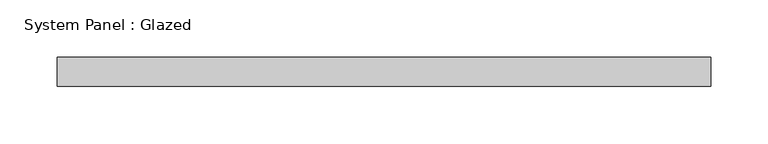
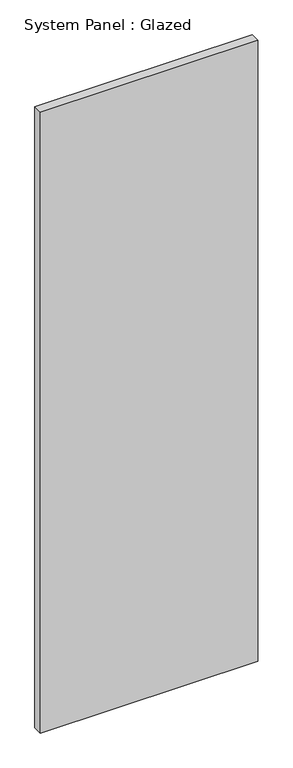
"""IFC4 building model written with IfcOpenShell, lengths in millimetres: plate geometry, System Panel : Glazed."""

from ifc_helpers import new_model, si_unit, origin, origin_with_axes, place, context, project, spatial, polyline, outline, extrude, source, transform, mapped, element, save


def system_panel_glazed_76ec949d(model_context):
    return source(origin(), model_context, "Body", "SweptSolid", [
        extrude(outline(polyline([(285.75, -44.45), (-285.75, -44.45), (-285.75, -19.05), (285.75, -19.05), (285.75, -44.45)])), origin_with_axes(), (0.0, 0.0, 1.0), 1727.2),
    ])


if __name__ == "__main__":
    model = new_model("IFC4")
    model_context = context("Model", 3, world=origin())
    ifc_project = project(units=[si_unit("LENGTHUNIT", "METRE", prefix="MILLI")], contexts=[model_context])
    site = spatial("IfcSite", under=ifc_project)
    building = spatial("IfcBuilding", under=site)
    placement = place(None, origin())
    system_panel_glazed_shape = system_panel_glazed_76ec949d(model_context)
    element("IfcPlate", 1, ObjectType="System Panel : Glazed", at=placement, inside=building, context=model_context, shape_type="MappedRepresentation", body=[
        mapped(system_panel_glazed_shape, transform((0.0, 0.0, 0.0), x_axis=(1.0, 0.0, 0.0), y_axis=(0.0, 1.0, 0.0), z_axis=(0.0, 0.0, 1.0))),
    ])
    save(model, "model.ifc")

# Revit data of these elements
# Type "System Panel : Glazed"
#   Construction Type Id = "GSP4R"
#   Analytic Construction = "1/8 in Pilkington single glazing"
#   Visual Light Transmittance = 0.9
#   Solar Heat Gain Coefficient = 0.86
#   Heat Transfer Coefficient (U) = 1.18115 BTU/(h·ft²·°F)
#   Define Thermal Properties by = 1
# Element 1 (IfcPlate, "System Panel : Glazed")
#   Materials on its faces: "Glass"
# Materials
#   "Glass": class "Glass", colour RGB 0 128 192, transparency 0.75, Description = "Soda Lime Glass", Cost = 0
